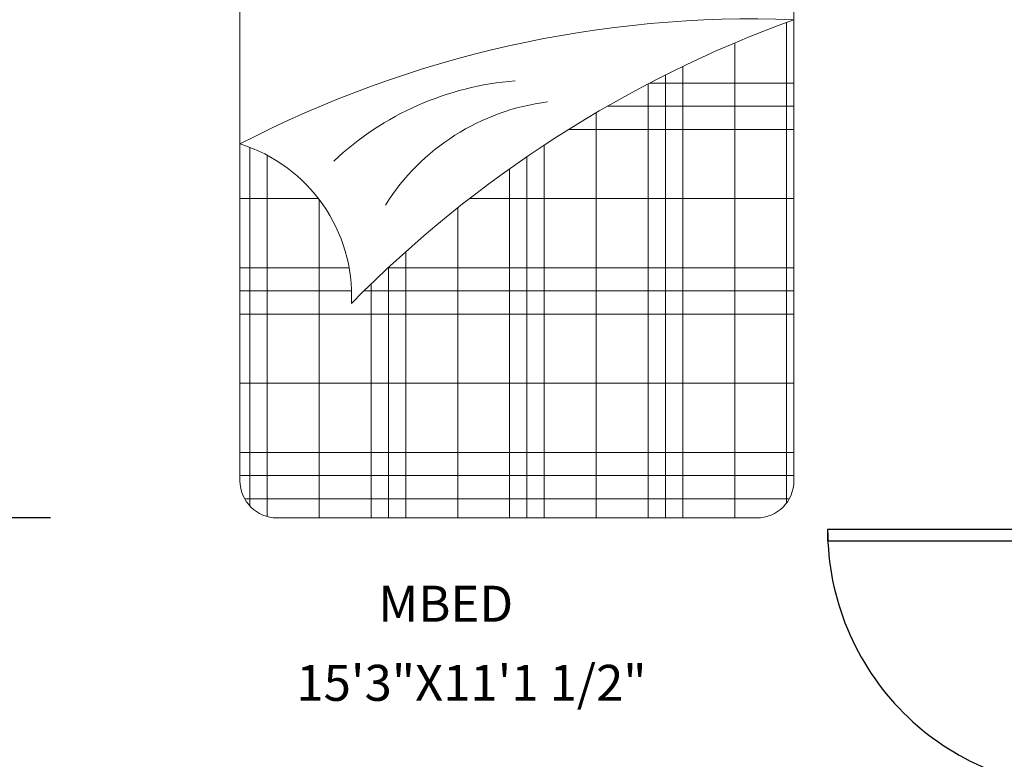
# Model space of a CAD drawing. Units: inches. Extents: x 3283068 to 3284536, y 3240756 to 3241803.
# Tile 9 of 19: x 3283383 to 3283520, y 3241501 to 3241603. Entities that reach past the tile are written whole.
import ezdxf

# ---------------------------------------------------------------- set-up
doc = ezdxf.new("R2010")
doc.units = ezdxf.units.IN
for name, color, linetype, lineweight in [('A-ANNO-DIMS', 2, 'Continuous', 18), ('A-AREA-IDEN', 7, 'Continuous', 18), ('door', 140, 'Continuous', 25), ('furniture', 40, 'Continuous', 18)]:
    doc.layers.add(name, color=color, linetype=linetype, lineweight=lineweight)
doc.styles.get("Standard").update_dxf_attribs({"font": 'arial.ttf'})
doc.dimstyles.new('ISO-25', dxfattribs={"dimtxt": 5, "dimasz": 2.5, "dimexe": 1.25, "dimexo": 0.625, "dimtad": 1, "dimlunit": 4, "dimtxsty": 'Standard', "dimblk": 'ARCHTICK', "dimcen": 2.5, "dimadec": 0, "dimazin": 0, "dimtfac": 1, "dimtmove": 0, "dimatfit": 3, "dimfxl": 1, "dimarcsym": 0})

# ---------------------------------------------------------------- blocks, each defined once
blk = doc.blocks.new('*U7')
for p, q in [((0, 0), (0, 6)), ((40, 0), (40, 6))]:
    blk.add_line(p, q)
blk.add_lwpolyline([(0, 0), (0, -40), (1.75, -40), (1.75, 0)], close=True)
blk.add_arc((0, 0), 40, 270, 0)
blk = doc.blocks.new('*X10')
at = {"color": 0}
for p, q in [((276.598, 451.25), (280.51, 451.25)), ((275.455, 450.625), (280.51, 450.625)), ((274.411, 450), (280.51, 450)), ((265.51, 448.125), (267.634, 448.125)), ((271.723, 448.125), (280.51, 448.125)), ((265.51, 446.25), (268.465, 446.25)), ((269.519, 446.25), (280.51, 446.25)), ((265.51, 445.625), (268.531, 445.625)), ((268.866, 445.625), (280.51, 445.625)), ((265.51, 445), (280.51, 445)), ((265.51, 443.125), (280.51, 443.125)), ((265.51, 441.25), (280.51, 441.25)), ((265.51, 440.625), (280.51, 440.625)), ((265.634, 440), (280.386, 440))]:
    blk.add_line(p, q, dxfattribs=at)
blk = doc.blocks.new('*X11')
at = {"color": 0}
for p, q in [((280.312, 439.886), (280.312, 452.896)), ((278.906, 439.482), (278.906, 452.338)), ((277.5, 439.482), (277.5, 451.702)), ((277.031, 439.482), (277.031, 451.471)), ((276.562, 439.482), (276.562, 451.231)), ((275.156, 439.482), (275.156, 450.451)), ((273.75, 439.482), (273.75, 449.576)), ((265.781, 439.797), (265.781, 449.511)), ((266.25, 439.517), (266.25, 449.296)), ((273.281, 439.482), (273.281, 449.261)), ((272.812, 439.482), (272.812, 448.934)), ((267.656, 439.482), (267.656, 448.095)), ((271.406, 439.482), (271.406, 447.876)), ((270, 439.482), (270, 446.689)), ((269.531, 439.482), (269.531, 446.262)), ((269.062, 439.482), (269.062, 445.817))]:
    blk.add_line(p, q, dxfattribs=at)
blk = doc.blocks.new('A$C52E67D0D')
at = {"layer": 'furniture'}
blk.add_lwpolyline([(1901, 0), (601, 0, -0.414214), (501, 100), (501, 1700, -0.414214), (601, 1800), (1901, 1800, -0.414214), (2001, 1700), (2001, 100, -0.414214)], format="xyb", close=True, dxfattribs=at)
for centre, radius, start, end in [((1888.6, -1664.5), 3015.3, 87.8642, 117.4001), ((3101, -1685.8), 3227.7, 109.926, 135.3977), ((1308.8, 377.9), 807.6, 94.4436, 133.2788), ((1410.8, 520.2), 610.8, 97.2157, 147.6656), ((371.4, 600.4), 432, 357.3792, 72.5379)]:
    blk.add_arc(centre, radius, start, end, dxfattribs=at)
at = {"layer": 'furniture', "xscale": 100, "yscale": 100, "zscale": 100}
for name in ['*X11', '*X10']:
    blk.add_blockref(name, (-26050, -43948.2), dxfattribs=at)
blk = doc.blocks.new('_ArchTick')
at = {"color": 0, "linetype": 'ByBlock', "const_width": 0.15}
blk.add_lwpolyline([(-0.5, -0.5), (0.5, 0.5)], dxfattribs=at)
blk = doc.blocks.new('*D58')
at = {"layer": 'A-ANNO-DIMS', "color": 0, "lineweight": -2, "transparency": 16777216}
for p, q in [((3283387.6, 3241626.59), (3283367.72, 3241626.59)), ((3283368.97, 3241534.23), (3283368.97, 3241626.59)), ((3283387.6, 3241534.23), (3283367.72, 3241534.23))]:
    blk.add_line(p, q, dxfattribs=at)
at = {"layer": 'Defpoints', "color": 0, "transparency": 16777216}
for p in [(3283368.97, 3241626.59), (3283388.23, 3241626.59), (3283388.23, 3241534.23)]:
    blk.add_point(p, dxfattribs=at)
at = {"layer": 'A-ANNO-DIMS', "color": 0, "lineweight": -2, "transparency": 16777216, "xscale": 2.5, "yscale": 2.5, "zscale": 2.5}
for p, rotation in [((3283368.97, 3241626.59), 90), ((3283368.97, 3241534.23), 270)]:
    blk.add_blockref('_ArchTick', p, dxfattribs=dict(at, rotation=rotation))
at = {"layer": 'A-ANNO-DIMS', "color": 0, "transparency": 16777216, "insert": (3283365.76, 3241580.41), "char_height": 5, "attachment_point": 5, "rotation": 90}
blk.add_mtext('7\'-8 1/2"', dxfattribs=at)
blk = doc.blocks.new('*D63')
at = {"layer": 'A-ANNO-DIMS', "color": 0, "lineweight": -2, "transparency": 16777216}
for p, q in [((3283248.09, 3241083.23), (3283248.09, 3241798.08)), ((3284328.09, 3241083.23), (3284328.09, 3241798.08)), ((3283248.09, 3241796.83), (3284328.09, 3241796.83))]:
    blk.add_line(p, q, dxfattribs=at)
at = {"layer": 'Defpoints', "color": 0, "transparency": 16777216}
for p in [(3284328.09, 3241796.83), (3283248.09, 3241082.6), (3284328.09, 3241082.6)]:
    blk.add_point(p, dxfattribs=at)
at = {"layer": 'A-ANNO-DIMS', "color": 0, "lineweight": -2, "transparency": 16777216, "xscale": 2.5, "yscale": 2.5, "zscale": 2.5, "rotation": 180}
blk.add_blockref('_ArchTick', (3283248.09, 3241796.83), dxfattribs=at)
at = {"layer": 'A-ANNO-DIMS', "color": 0, "lineweight": -2, "transparency": 16777216, "xscale": 2.5, "yscale": 2.5, "zscale": 2.5}
blk.add_blockref('_ArchTick', (3284328.09, 3241796.83), dxfattribs=at)
at = {"layer": 'A-ANNO-DIMS', "color": 0, "transparency": 16777216, "insert": (3283788.09, 3241800.01), "char_height": 5, "attachment_point": 5}
blk.add_mtext('90\'-0"', dxfattribs=at)

msp = doc.modelspace()

# ---------------------------------------------------------------- block references
at = {"layer": 'door', "xscale": 0.9, "yscale": 0.9, "zscale": 0.9, "rotation": 270}
msp.add_blockref('*U7', (3283531.589, 3241532.602), dxfattribs=at)
at = {"layer": 'furniture', "xscale": 0.0513129658560468, "yscale": 0.0513129658560468, "zscale": 0.0513129658560468}
msp.add_blockref('A$C52E67D0D', (3283388.229, 3241534.227), dxfattribs=at)

# ---------------------------------------------------------------- texts
at = {"layer": 'A-AREA-IDEN'}
for s, p in [('        MBED', (3283420.939, 3241519.8)), ('15\'3"X11\'1 1/2"', (3283421.776, 3241508.81))]:
    msp.add_text(s, height=5, dxfattribs=at).set_placement(p)

# ---------------------------------------------------------------- dimensions: what is measured, and where the dimension line sits
at = {"layer": 'A-ANNO-DIMS'}
dim = msp.add_linear_dim(base=(3284328.089, 3241796.827), p1=(3283248.089, 3241082.602), p2=(3284328.089, 3241082.602), dimstyle='ISO-25', override={"dimdec": 1, "dimlfac": 1, "dimrnd": 0, "dimzin": 1, "dimdsep": 46, "dimlunit": 4, "dimfrac": 2}, dxfattribs=at)
dim.commit()
dim.dimension.update_dxf_attribs({"geometry": '*D63', "text_midpoint": (3283788.089, 3241800.005)})
dim = msp.add_linear_dim(base=(3283368.971, 3241626.59), p1=(3283388.229, 3241534.227), p2=(3283388.229, 3241626.59), angle=90, dimstyle='ISO-25', override={"dimdec": 1, "dimlfac": 1, "dimrnd": 0, "dimzin": 1, "dimdsep": 46, "dimlunit": 4, "dimfrac": 2}, dxfattribs=at)
dim.commit()
dim.dimension.update_dxf_attribs({"geometry": '*D58', "text_midpoint": (3283365.761, 3241580.409)})

doc.saveas('drawing.dxf')
